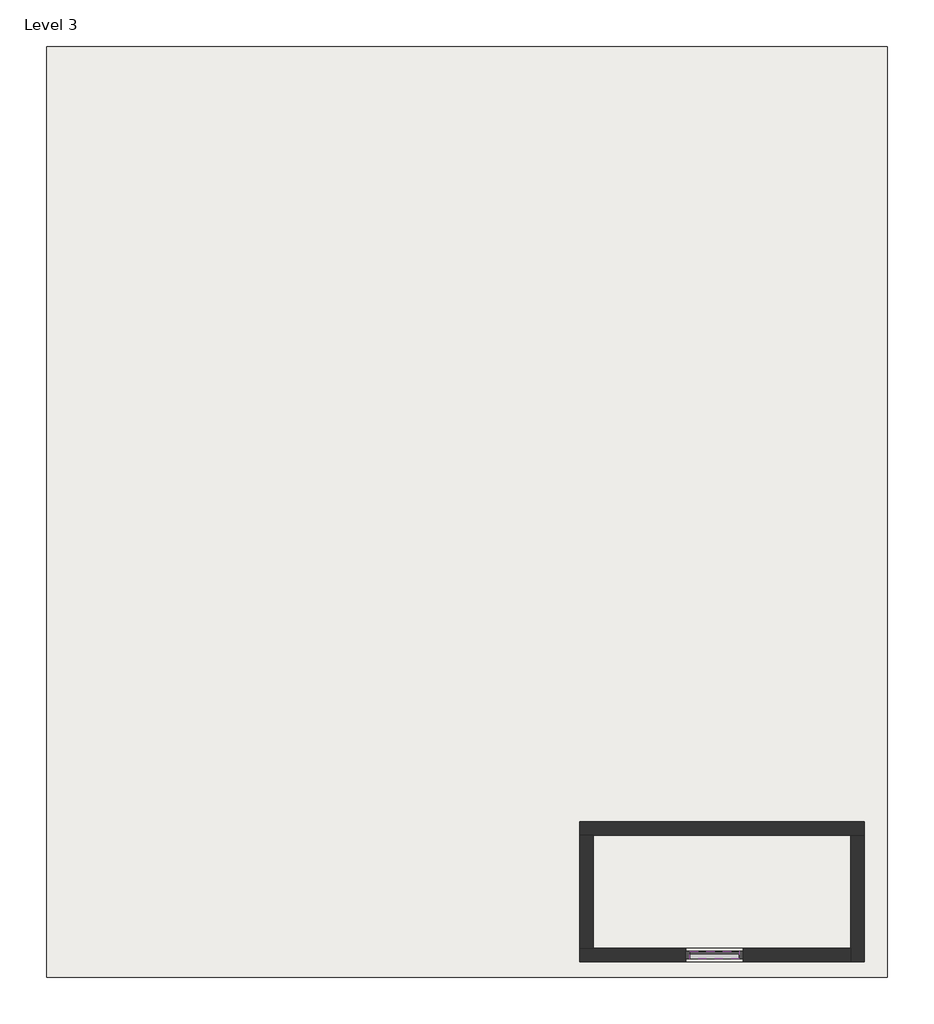
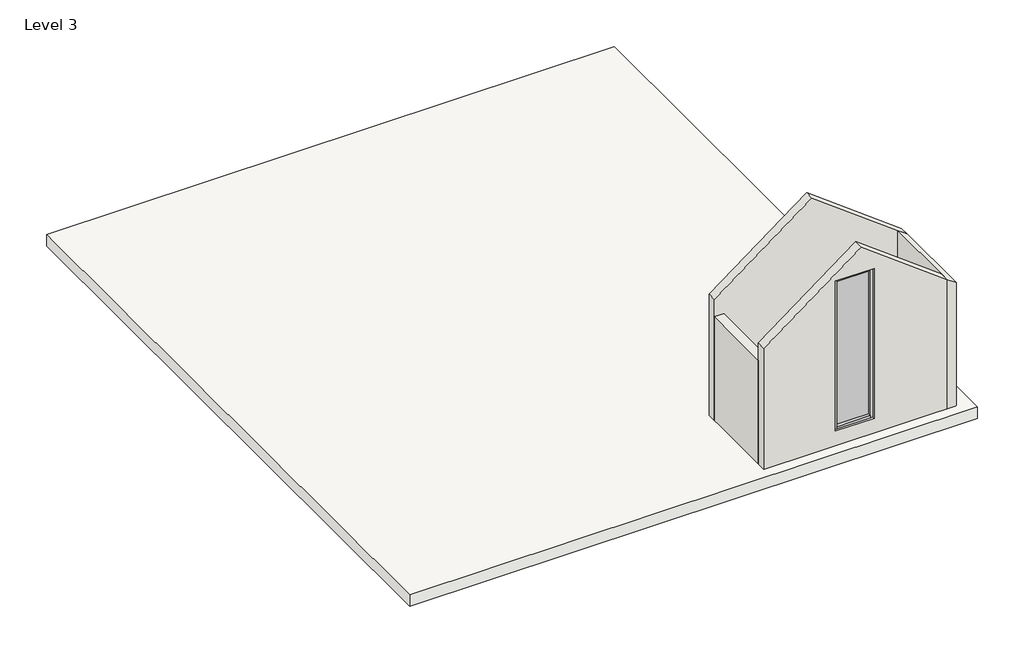
# One storey: 4 members, 4 walls, 1 plate, 1 roof.
"""IFC4 building model written with IfcOpenShell, lengths in millimetres."""

from ifc_helpers import new_model, si_unit, frame, origin, place, context, project, spatial, polyline, outline, extrude, faceted_brep, transform, mapped, element, save
from components import member_86adc6a2, member_ab6d823a, system_panel_glazed_20744f22

model = new_model("IFC4")

# Units and contexts
model_context = context("Model", 3, world=origin())
ifc_project = project(units=[si_unit("LENGTHUNIT", "METRE", prefix="MILLI")], contexts=[model_context])

# Site, building, storey
site = spatial("IfcSite", under=ifc_project)
building = spatial("IfcBuilding", under=site)
storey = spatial("IfcBuildingStorey", under=building, Name="Level 3", Elevation=6096.0)

# Members
placement = place(None, origin())
member_shape = member_86adc6a2(model_context)
element("IfcMember", 1, ObjectType="Rectangular Mullion : 2.5\" x 5\" rectangular", at=placement, inside=storey, context=model_context, shape_type="MappedRepresentation", body=[
    mapped(member_shape, transform((-7505.1403308, -12974.3518738, 10745.481127), x_axis=(0.0, 0.0, 1.0), y_axis=(0.0, -1.0, 0.0), z_axis=(1.0, 0.0, 0.0))),
])
element("IfcMember", 2, ObjectType="Rectangular Mullion : 2.5\" x 5\" rectangular", at=placement, inside=storey, context=model_context, shape_type="MappedRepresentation", body=[
    mapped(member_shape, transform((-8343.3403308, -12974.3518738, 6787.2360632), x_axis=(0.0, 0.0, -1.0), y_axis=(0.0, -1.0, 0.0), z_axis=(-1.0, 0.0, 0.0))),
])
member_2_shape = member_ab6d823a(model_context)
element("IfcMember", 3, ObjectType="Rectangular Mullion : 2.5\" x 5\" rectangular", at=placement, inside=storey, context=model_context, shape_type="MappedRepresentation", body=[
    mapped(member_2_shape, transform((-8406.8403308, -12974.3518738, 10745.481127), x_axis=(-1.0, 0.0, 0.0), y_axis=(0.0, -1.0, 0.0), z_axis=(0.0, 0.0, 1.0))),
])
element("IfcMember", 4, ObjectType="Rectangular Mullion : 2.5\" x 5\" rectangular", at=placement, inside=storey, context=model_context, shape_type="MappedRepresentation", body=[
    mapped(member_2_shape, transform((-7441.6403308, -12974.3518738, 6787.2360632), x_axis=(1.0, 0.0, 0.0), y_axis=(0.0, -1.0, 0.0), z_axis=(0.0, 0.0, -1.0))),
])

# Plate
system_panel_glazed_shape = system_panel_glazed_20744f22(model_context)
element("IfcPlate", 5, ObjectType="System Panel : Glazed", at=placement, inside=storey, context=model_context, shape_type="MappedRepresentation", body=[
    mapped(system_panel_glazed_shape, transform((-7924.2403308, -12974.3518738, 6850.7360632), x_axis=(1.0, 0.0, 0.0), y_axis=(0.0, 1.0, 0.0), z_axis=(0.0, 0.0, 1.0))),
])

# Roof
element("IfcRoof", 6, ObjectType="Generic - 12\"", at=placement, inside=storey, context=model_context, shape_type="SweptSolid", body=[
    extrude(outline(polyline([(-19189.1403308, 2341.8481262), (-5015.9403308, 2341.8481262), (-5015.9403308, -13355.3518738), (-19189.1403308, -13355.3518738), (-19189.1403308, 2341.8481262)])), frame((0.0, 0.0, 6096.0), z_axis=(0.0, 0.0, 1.0), x_axis=(1.0, 0.0, 0.0)), (0.0, 0.0, 1.0), 304.8),
])

# Walls
element("IfcWall", 7, ObjectType="9\"", at=placement, inside=storey, context=model_context, shape_type="Brep", body=[
    faceted_brep([(-10197.5403308, -10955.0518738, 6096.0), (-9968.9403308, -10955.0518738, 6096.0), (-5625.5403308, -10955.0518738, 6096.0), (-5396.9403308, -10955.0518738, 6096.0), (-5396.9403308, -10955.0518738, 9651.5527957), (-5625.5403308, -10955.0518738, 9823.0027957), (-7762.503675, -10955.0518738, 11425.7253039), (-10197.5403308, -10955.0518738, 9599.4478121), (-10197.5403308, -10955.0518738, 9144.0), (-10197.5403308, -10726.4518738, 6096.0), (-10197.5403308, -10726.4518738, 9599.4478121), (-7762.503675, -10726.4518738, 11425.7253039), (-5396.9403308, -10726.4518738, 9651.5527957), (-5396.9403308, -10726.4518738, 6096.0)], [[[0, 1, 2, 3, 4, 5, 6, 7, 8]], [[9, 10, 11, 12, 13]], [[3, 2, 1, 0, 9, 13]], [[4, 3, 13, 12]], [[0, 8, 7, 10, 9]], [[7, 6, 11, 10]], [[6, 5, 4, 12, 11]]]),
])
element("IfcWall", 8, ObjectType="9\"", at=placement, inside=storey, context=model_context, shape_type="Brep", body=[
    faceted_brep([(-5625.5403308, -10955.0518738, 6096.0), (-5625.5403308, -12860.0518738, 6096.0), (-5625.5403308, -13088.6518738, 6096.0), (-5625.5403308, -13088.6518738, 9823.0027957), (-5625.5403308, -12860.0518738, 9823.0027957), (-5625.5403308, -10955.0518738, 9823.0027957), (-5396.9403308, -10955.0518738, 6096.0), (-5396.9403308, -10955.0518738, 9651.5527957), (-5396.9403308, -13088.6518738, 9651.5527957), (-5396.9403308, -13088.6518738, 6096.0)], [[[0, 1, 2, 3, 4, 5]], [[6, 7, 8, 9]], [[2, 1, 0, 6, 9]], [[0, 5, 7, 6]], [[3, 2, 9, 8]], [[5, 4, 3, 8, 7]]]),
])
element("IfcWall", 9, ObjectType="9\"", at=placement, inside=storey, context=model_context, shape_type="Brep", body=[
    faceted_brep([(-5625.5403308, -12860.0518738, 6096.0), (-9968.9403308, -12860.0518738, 6096.0), (-10197.5403308, -12860.0518738, 6096.0), (-10197.5403308, -12860.0518738, 9144.0), (-10197.5403308, -12860.0518738, 9599.4478121), (-7762.503675, -12860.0518738, 11425.7253039), (-5625.5403308, -12860.0518738, 9823.0027957), (-8406.8403308, -12860.0518738, 10745.481127), (-8406.8403308, -12860.0518738, 6787.2360632), (-7441.6403308, -12860.0518738, 6787.2360632), (-7441.6403308, -12860.0518738, 10745.481127), (-10197.5403308, -13088.6518738, 6096.0), (-5625.5403308, -13088.6518738, 6096.0), (-5625.5403308, -13088.6518738, 9823.0027957), (-7762.503675, -13088.6518738, 11425.7253039), (-10197.5403308, -13088.6518738, 9599.4478121), (-8406.8403308, -13088.6518738, 6787.2360632), (-8406.8403308, -13088.6518738, 10745.481127), (-7441.6403308, -13088.6518738, 10745.481127), (-7441.6403308, -13088.6518738, 6787.2360632)], [[[0, 1, 2, 3, 4, 5, 6], [7, 8, 9, 10]], [[11, 12, 13, 14, 15], [16, 17, 18, 19]], [[2, 1, 0, 12, 11]], [[0, 6, 13, 12]], [[4, 3, 2, 11, 15]], [[13, 6, 5, 14]], [[4, 15, 14, 5]], [[16, 8, 7, 17]], [[17, 7, 10, 18]], [[18, 10, 9, 19]], [[8, 16, 19, 9]]]),
])
element("IfcWall", 10, ObjectType="9\"", at=placement, inside=storey, context=model_context, shape_type="SweptSolid", body=[
    extrude(outline(polyline([(-10197.5403308, -12860.0518738), (-10197.5403308, -10955.0518738), (-9968.9403308, -10955.0518738), (-9968.9403308, -12860.0518738), (-10197.5403308, -12860.0518738)])), frame((0.0, 0.0, 6096.0), z_axis=(0.0, 0.0, 1.0), x_axis=(1.0, 0.0, 0.0)), (0.0, 0.0, 1.0), 3048.0),
])

save(model, "model.ifc")

# Revit data of these elements
# Type "Rectangular Mullion : 2.5\" x 5\" rectangular"
#   built-in parameter 1007304 = 0.416667 (stored number, unit not read)
#   built-in parameter 1007301 = 0.104167 (stored number, unit not read)
#   built-in parameter 1007300 = 0.104167 (stored number, unit not read)
# Type "System Panel : Glazed"
#   Construction Type Id = "GSP4R"
#   Analytic Construction = "1/8 in Pilkington single glazing"
#   Visual Light Transmittance = 0.9
#   Solar Heat Gain Coefficient = 0.86
#   Heat Transfer Coefficient (U) = 1.18115 BTU/(h·ft²·°F)
#   Define Thermal Properties by = 1
# Type "Generic - 12\""
#   Assembly Code = "B1020"
#   Layers, outside or top first: 1' - 0" no material (function 1)
# Type "9\""
#   Assembly Code = "B2010"
#   Layers, outside or top first: 0' - 9" no material (function 1)
# Elements 1, 2, 3, 4 (IfcMember, "Rectangular Mullion : 2.5\" x 5\" rectangular")
#   Phase Created = New Construction
#   Materials on its faces: "Aluminum"
# Element 5 (IfcPlate, "System Panel : Glazed")
#   Phase Created = New Construction
#   Materials on its faces: "Glass"
# Element 6 (IfcRoof, "Generic - 12\"")
#   built-in parameter 1001705 = 21 (stored number, unit not read)
#   built-in parameter 1001710 = 33615
#   Phase Created = New Construction
#   Materials on its faces: "Default Roof"
# Elements 7, 8, 9, 10 (IfcWall, "9\"")
#   Top Offset = 0' - 0"
#   Base Offset = 0' - 0"
#   Unconnected Height = 10' - 0"
#   wall height = 10' - 0"
#   Phase Created = New Construction
#   Base Constraint = Level 3
#   Materials on its faces: "Default Wall"
# Materials
#   "Aluminum": class "Metal", colour RGB 247 247 247, transparency 0, Description = "Aluminum 6061", Cost = 0
#   "Glass": class "Glass", colour RGB 0 128 192, transparency 0.75, Description = "Soda Lime Glass", Cost = 0
#   "Default Roof": colour RGB 88 101 114, transparency 0, Cost = 0
#   "Default Wall": colour RGB 128 128 128, transparency 0, Cost = 0
